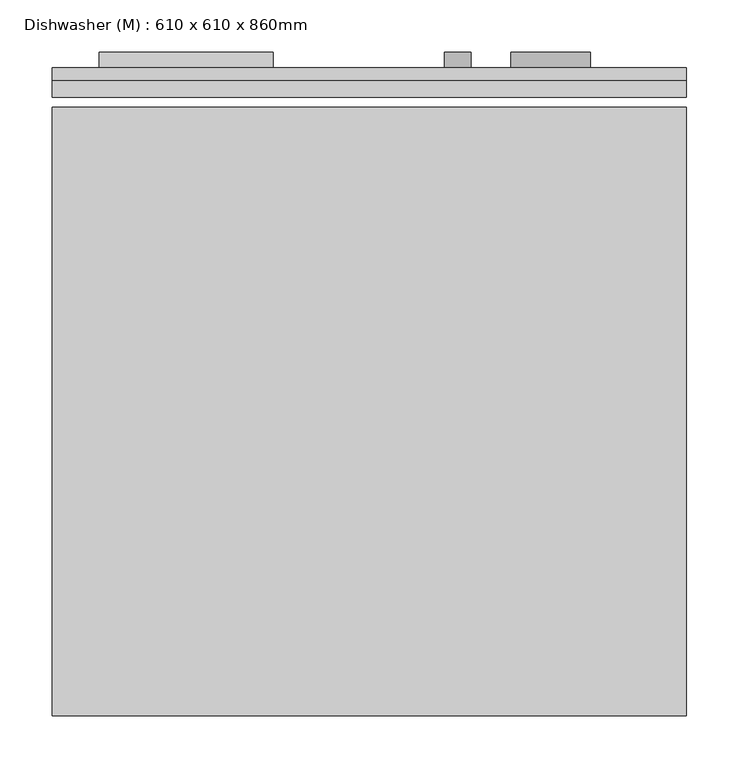
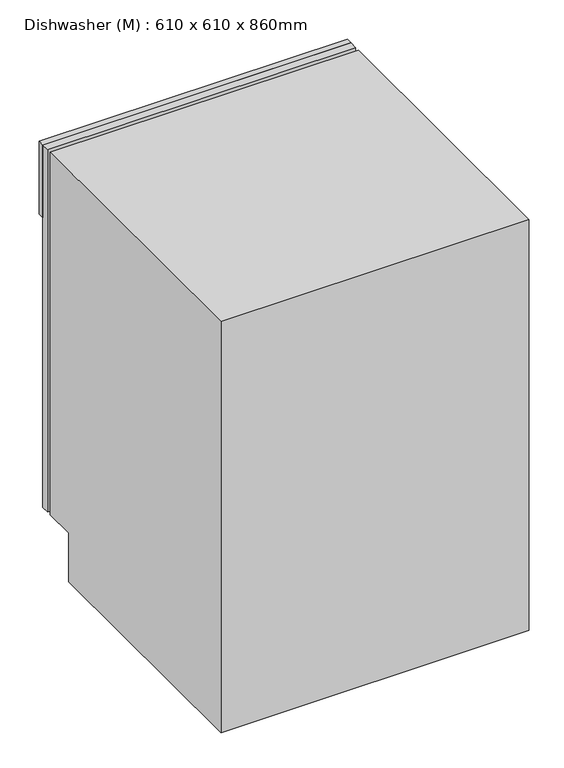
"""IFC4 building model written with IfcOpenShell, lengths in millimetres: proxy geometry, Dishwasher (M) : 610 x 610 x 860mm."""

from ifc_helpers import new_model, si_unit, point, frame, frame_2d, origin, place, context, project, spatial, polyline, circle_curve, trimmed, segment, composite_curve, outline, extrude, source, transform, mapped, element, save


def dishwasher_m_610_x_610_x_860mm_59039f12(model_context):
    return source(origin(), model_context, "Body", "SweptSolid", [
        extrude(outline(polyline([(687.5174685, 38.3504352), (687.5174685, 22.4754352), (77.5174685, 22.4754352), (77.5174685, 38.3504352), (687.5174685, 38.3504352)])), frame((0.0, 0.0, 101.6), z_axis=(0.0, 0.0, 1.0), x_axis=(1.0, 0.0, 0.0)), (0.0, 0.0, 1.0), 758.4),
        extrude(outline(polyline([(687.5174685, 38.3504352), (77.5174685, 38.3504352), (77.5174685, 51.0504352), (687.5174685, 51.0504352), (687.5174685, 38.3504352)])), frame((0.0, 0.0, 707.6), z_axis=(0.0, 0.0, 1.0), x_axis=(1.0, 0.0, 0.0)), (0.0, 0.0, 1.0), 152.4),
        extrude(outline(polyline([(-571.6495648, 0.0), (-571.6495648, 860.0), (12.9504352, 860.0), (12.9504352, 101.6), (-50.5495648, 101.6), (-50.5495648, 0.0), (-571.6495648, 0.0)])), frame((77.5174685, 0.0, 0.0), z_axis=(1.0, 0.0, 0.0), x_axis=(0.0, 1.0, 0.0)), (0.0, 0.0, 1.0), 610.0),
        extrude(outline(polyline([(290.2347603, 66.0504352), (290.2347603, 51.0504352), (122.8347603, 51.0504352), (122.8347603, 66.0504352), (290.2347603, 66.0504352)])), frame((0.0, 0.0, 775.6663551), z_axis=(0.0, 0.0, 1.0), x_axis=(1.0, 0.0, 0.0)), (0.0, 0.0, 1.0), 50.8),
        extrude(outline(composite_curve([segment(trimmed(circle_curve(frame_2d((775.6663551, 467.3393328)), 12.7), [point((775.6663551, 480.0393328))], [point((775.6663551, 454.6393328))], False, "CARTESIAN"), True, "CONTINUOUS"), segment(trimmed(circle_curve(frame_2d((775.6663551, 467.3393328)), 12.7), [point((775.6663551, 454.6393328))], [point((775.6663551, 480.0393328))], False, "CARTESIAN"), True, "CONTINUOUS")], self_intersect=False)), frame((0.0, 51.0504352, 0.0), z_axis=(0.0, 1.0, 0.0), x_axis=(0.0, 0.0, 1.0)), (0.0, 0.0, 1.0), 15.0),
        extrude(outline(composite_curve([segment(trimmed(circle_curve(frame_2d((775.6663551, 556.7855874)), 38.1), [point((775.6663551, 594.8855874))], [point((775.6663551, 518.6855874))], False, "CARTESIAN"), True, "CONTINUOUS"), segment(trimmed(circle_curve(frame_2d((775.6663551, 556.7855874)), 38.1), [point((775.6663551, 518.6855874))], [point((775.6663551, 594.8855874))], False, "CARTESIAN"), True, "CONTINUOUS")], self_intersect=False)), frame((0.0, 51.0504352, 0.0), z_axis=(0.0, 1.0, 0.0), x_axis=(0.0, 0.0, 1.0)), (0.0, 0.0, 1.0), 15.0),
    ])


if __name__ == "__main__":
    model = new_model("IFC4")
    model_context = context("Model", 3, world=origin())
    ifc_project = project(units=[si_unit("LENGTHUNIT", "METRE", prefix="MILLI")], contexts=[model_context])
    site = spatial("IfcSite", under=ifc_project)
    building = spatial("IfcBuilding", under=site)
    placement = place(None, origin())
    dishwasher_m_610_x_610_x_860mm_shape = dishwasher_m_610_x_610_x_860mm_59039f12(model_context)
    element("IfcBuildingElementProxy", 1, Name="Dishwasher (M) : 610 x 610 x 860mm", ObjectType="Dishwasher (M) : 610 x 610 x 860mm", at=placement, inside=building, context=model_context, shape_type="MappedRepresentation", body=[
        mapped(dishwasher_m_610_x_610_x_860mm_shape, transform((0.0, 0.0, 0.0), x_axis=(1.0, 0.0, 0.0), y_axis=(0.0, 1.0, 0.0), z_axis=(0.0, 0.0, 1.0))),
    ])
    save(model, "model.ifc")

# Revit data of these elements
# Type "Dishwasher (M) : 610 x 610 x 860mm"
#   Label = "DW"
#   Depth = 2' - 0.01575"
#   Height = 2' - 9.85827"
#   Width = 2' - 0.01575"
#   Dishwasher Material = Metal - Paint Finish - Ivory,Glossy
#   Panel Face Material = Plastic - Black
#   Default Elevation = 0
# Element 1 (IfcBuildingElementProxy, "Dishwasher (M) : 610 x 610 x 860mm")
#   Materials on its faces: "Metal - Paint Finish - Ivory,Glossy", "Plastic - Black"
# Materials
#   "Metal - Paint Finish - Ivory,Glossy": colour RGB 247 247 239, transparency 0
#   "Plastic - Black": colour RGB 0 0 0, transparency 0.7
